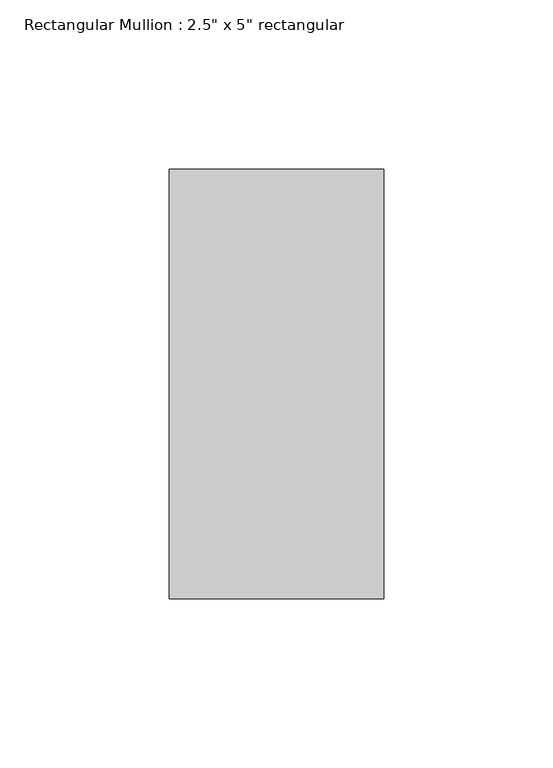
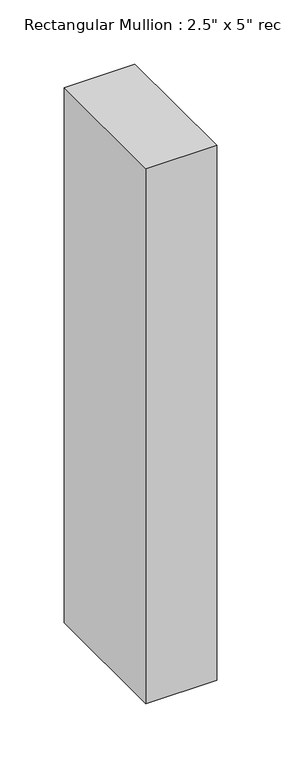
"""IFC4 building model written with IfcOpenShell, lengths in millimetres: member geometry."""

from ifc_helpers import new_model, si_unit, frame, origin, place, context, project, spatial, polyline, outline, extrude, source, transform, mapped, element, save


def member_90750a43(model_context):
    return source(origin(), model_context, "Body", "SweptSolid", [
        extrude(outline(polyline([(31.75, 63.5), (31.75, -63.5), (-31.75, -63.5), (-31.75, 63.5), (31.75, 63.5)])), frame((0.0, 0.0, -508.0), z_axis=(0.0, 0.0, 1.0), x_axis=(1.0, 0.0, 0.0)), (0.0, 0.0, 1.0), 508.0),
    ])


if __name__ == "__main__":
    model = new_model("IFC4")
    model_context = context("Model", 3, world=origin())
    ifc_project = project(units=[si_unit("LENGTHUNIT", "METRE", prefix="MILLI")], contexts=[model_context])
    site = spatial("IfcSite", under=ifc_project)
    building = spatial("IfcBuilding", under=site)
    placement = place(None, origin())
    member_shape = member_90750a43(model_context)
    element("IfcMember", 1, ObjectType="Rectangular Mullion : 2.5\" x 5\" rectangular", at=placement, inside=building, context=model_context, shape_type="MappedRepresentation", body=[
        mapped(member_shape, transform((0.0, 0.0, 0.0), x_axis=(1.0, 0.0, 0.0), y_axis=(0.0, 1.0, 0.0), z_axis=(0.0, 0.0, 1.0))),
    ])
    save(model, "model.ifc")

# Revit data of these elements
# Type "Rectangular Mullion : 2.5\" x 5\" rectangular"
#   built-in parameter 1007304 = 0.416667 (stored number, unit not read)
#   built-in parameter 1007301 = 0.104167 (stored number, unit not read)
#   built-in parameter 1007300 = 0.104167 (stored number, unit not read)
# Element 1 (IfcMember, "Rectangular Mullion : 2.5\" x 5\" rectangular")
#   Materials on its faces: "door colour"
# Materials
#   "door colour": class "Generic", colour RGB 120 120 120, transparency 0, Cost = 0
